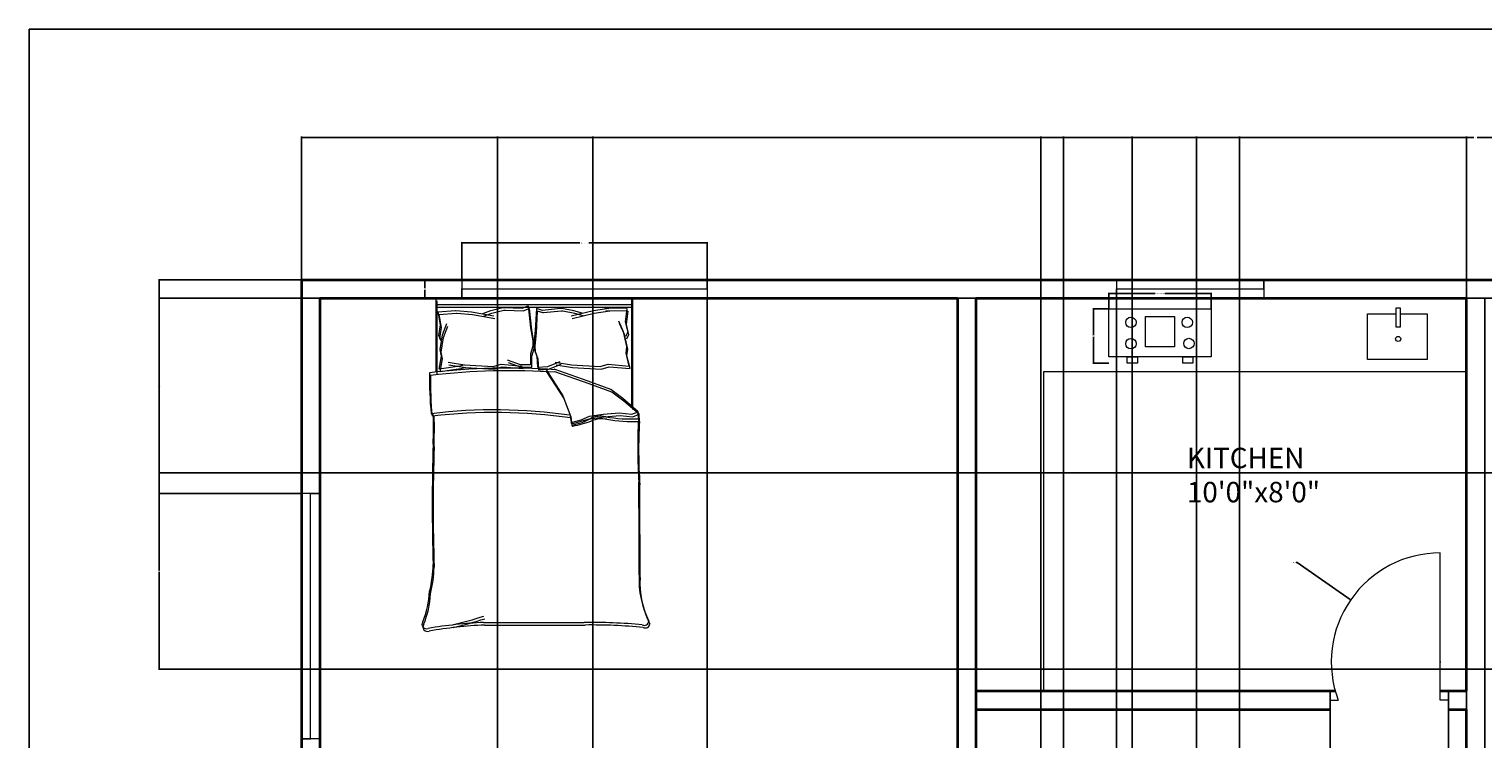
# Model space of a CAD drawing. Units: inches. Extents: x 1861 to 2564, y 1482 to 2317.
# Tile 7 of 11: x 1861 to 2217, y 2143 to 2317. Entities that reach past the tile are written whole.
import ezdxf

# ---------------------------------------------------------------- set-up
doc = ezdxf.new("R2010")
doc.units = ezdxf.units.IN
for name, color, linetype, lineweight in [('A-ANNO-DIMS', 2, 'Continuous', 18), ('A-ANNO-TTLB', 7, 'Continuous', 25), ('A-AREA-IDEN', 7, 'Continuous', 18), ('A-DOOR', 3, 'Continuous', 18), ('A-EQPM', 8, 'Continuous', 18), ('A-FLOR-CASE', 9, 'Continuous', 18), ('A-FLOR-FIXT', 8, 'Continuous', 18), ('A-FURN', 8, 'Continuous', 13), ('A-GLAZ', 4, 'Continuous', 18), ('A-WALL', 7, 'Continuous', 35)]:
    doc.layers.add(name, color=color, linetype=linetype, lineweight=lineweight)
doc.styles.get("Standard").update_dxf_attribs({"font": 'arial.ttf'})
doc.dimstyles.get("Standard").update_dxf_attribs({"dimtxt": 0.18, "dimasz": 0.18, "dimexe": 0.18, "dimexo": 0.0625, "dimgap": 0.09, "dimtad": 0, "dimtih": 1, "dimtoh": 1, "dimdec": 4, "dimzin": 0, "dimdsep": 46, "dimtxsty": 'Standard', "dimcen": 0.09, "dimadec": 0, "dimazin": 0, "dimtfac": 1, "dimtdec": 4, "dimtofl": 0, "dimtmove": 0, "dimatfit": 3, "dimfxl": 1, "dimtolj": 1, "dimtzin": 0, "dimarcsym": 0})

# ---------------------------------------------------------------- blocks, each defined once
blk = doc.blocks.new('WIN-60IN')
for p, q in [((0, 4.5), (0, 0)), ((60, 2.25), (60, 4.5)), ((60, 4.5), (60, 0)), ((0, 0), (0, 2.25)), ((0, 2.25), (60, 2.25))]:
    blk.add_line(p, q)
blk = doc.blocks.new('WIN-36IN')
for p, q in [((0, 4.5), (0, 0)), ((36, 2.25), (36, 4.5)), ((36, 4.5), (36, 0)), ((0, 0), (0, 2.25)), ((0, 2.25), (36, 2.25))]:
    blk.add_line(p, q)
blk = doc.blocks.new('BED-DOUBLE')
for p, q in [((3.48, 63.34), (3.48, 81.45)), ((3.48, 63.34), (3.48, 81.45)), ((51.27, 81.45), (3.48, 81.45)), ((3.48, 79.91), (51.27, 79.91)), ((3.48, 79.91), (51.27, 79.91)), ((3.7, 62.7), (3.7, 80.81)), ((3.7, 62.7), (3.7, 80.81)), ((3.7, 79.27), (51.49, 79.27)), ((3.7, 79.27), (51.49, 79.27)), ((3.9, 78.11), (8.18, 78.44)), ((3.9, 78.11), (8.18, 78.44)), ((8.18, 78.44), (8.29, 78.42)), ((8.18, 78.44), (8.29, 78.42)), ((8.29, 78.42), (12.11, 78.13)), ((8.29, 78.42), (12.11, 78.13)), ((14.86, 77.7), (16.88, 78.42)), ((14.86, 77.7), (16.88, 78.42)), ((16.88, 78.42), (19.77, 79.14)), ((16.88, 78.42), (19.77, 79.14)), ((17.11, 77.78), (20, 78.5)), ((17.11, 77.78), (20, 78.5)), ((19.77, 79.14), (20.09, 79.14)), ((19.77, 79.14), (20.09, 79.14)), ((20, 78.5), (20.32, 78.5)), ((20, 78.5), (20.32, 78.5)), ((20.09, 79.14), (24.54, 79)), ((20.09, 79.14), (24.54, 79)), ((20.32, 78.5), (24.77, 78.36)), ((20.32, 78.5), (24.77, 78.36)), ((24.54, 79), (25.98, 79.58)), ((24.54, 79), (25.98, 79.58)), ((24.77, 78.36), (26.21, 78.94)), ((24.77, 78.36), (26.21, 78.94)), ((25.98, 79.58), (26.56, 74.23)), ((25.98, 79.58), (26.56, 74.23)), ((26.21, 78.94), (26.79, 73.59)), ((26.21, 78.94), (26.79, 73.59)), ((27.98, 78.95), (27.73, 73.58)), ((27.98, 78.95), (27.73, 73.58)), ((28.21, 78.31), (27.96, 72.94)), ((28.21, 78.31), (27.96, 72.94)), ((29.46, 78.47), (27.98, 78.95)), ((29.46, 78.47), (27.98, 78.95)), ((29.69, 77.83), (28.21, 78.31)), ((29.68, 77.83), (28.21, 78.31)), ((33.88, 78.89), (29.46, 78.47)), ((33.88, 78.89), (29.46, 78.47)), ((34.11, 78.25), (29.68, 77.83)), ((34.11, 78.25), (29.69, 77.83)), ((34.21, 78.91), (33.88, 78.89)), ((34.21, 78.91), (33.88, 78.89)), ((34.43, 78.27), (34.11, 78.25)), ((34.43, 78.27), (34.11, 78.25)), ((37.14, 78.37), (34.21, 78.91)), ((37.14, 78.37), (34.21, 78.91)), ((37.36, 77.73), (34.43, 78.27)), ((37.36, 77.73), (34.43, 78.27)), ((41.92, 78.38), (36.5, 77.02)), ((41.92, 78.38), (36.5, 77.02)), ((39.2, 77.77), (37.14, 78.37)), ((39.2, 77.77), (37.14, 78.37)), ((45.71, 78.9), (41.92, 78.38)), ((45.71, 78.9), (41.92, 78.38)), ((45.94, 78.26), (42.14, 77.74)), ((45.94, 78.26), (42.14, 77.74)), ((50.11, 78.89), (44.71, 78.99)), ((44.71, 78.99), (45.71, 78.9)), ((50.11, 78.89), (44.71, 78.99)), ((44.71, 78.99), (45.71, 78.9)), ((50.34, 78.25), (44.94, 78.35)), ((44.94, 78.35), (45.94, 78.26)), ((50.34, 78.25), (44.94, 78.35)), ((44.94, 78.35), (45.94, 78.26)), ((50.11, 78.89), (49.73, 75.68)), ((50.11, 78.89), (49.73, 75.68)), ((50.34, 78.25), (49.96, 75.04)), ((50.34, 78.25), (49.96, 75.04)), ((51.27, 81.45), (51.27, 54.84)), ((51.27, 81.45), (51.27, 54.84)), ((51.27, 81.45), (51.49, 81.45)), ((51.49, 81.45), (51.49, 80.81)), ((51.49, 80.81), (51.49, 54.2)), ((51.49, 80.81), (51.49, 54.2)), ((3.9, 78.13), (4.47, 74.95)), ((3.9, 78.13), (4.47, 74.95)), ((4.47, 74.95), (4.04, 72.35)), ((4.47, 74.95), (4.04, 72.35)), ((4.12, 77.49), (4.7, 74.31)), ((4.12, 77.49), (4.7, 74.31)), ((4.13, 77.47), (8.41, 77.8)), ((4.13, 77.47), (8.41, 77.8)), ((5.05, 72.49), (6.06, 75.24)), ((5.05, 72.49), (6.06, 75.24)), ((8.41, 77.8), (8.51, 77.78)), ((8.41, 77.8), (8.51, 77.78)), ((8.51, 77.78), (12.34, 77.49)), ((8.51, 77.78), (12.34, 77.49)), ((12.11, 78.13), (17.6, 77.12)), ((12.11, 78.13), (17.6, 77.12)), ((12.34, 77.49), (17.83, 76.48)), ((12.34, 77.49), (17.83, 76.48)), ((15.08, 77.06), (17.11, 77.78)), ((15.08, 77.06), (17.11, 77.78)), ((42.14, 77.74), (36.72, 76.38)), ((42.14, 77.74), (36.72, 76.38)), ((39.43, 77.13), (37.36, 77.73)), ((39.43, 77.13), (37.36, 77.73)), ((49.31, 73.19), (48.13, 75.87)), ((49.31, 73.19), (48.13, 75.87)), ((49.54, 72.55), (48.36, 75.23)), ((49.54, 72.55), (48.36, 75.23)), ((49.73, 75.68), (50.33, 73.11)), ((49.73, 75.68), (50.33, 73.11)), ((49.96, 75.04), (50.56, 72.47)), ((49.96, 75.04), (50.56, 72.47)), ((4.04, 72.35), (4.62, 71.33)), ((4.04, 72.35), (4.62, 71.33)), ((4.7, 74.31), (4.27, 71.71)), ((4.7, 74.31), (4.27, 71.71)), ((4.27, 71.71), (4.85, 70.69)), ((4.27, 71.71), (4.85, 70.69)), ((4.47, 68.88), (5.05, 72.49)), ((4.47, 68.88), (5.05, 72.49)), ((4.7, 68.24), (5.28, 71.85)), ((4.7, 68.24), (5.28, 71.85)), ((5.28, 71.85), (6.29, 74.6)), ((5.28, 71.85), (6.29, 74.6)), ((26.56, 74.23), (27.14, 71.04)), ((26.56, 74.23), (27.14, 71.04)), ((26.79, 73.59), (27.37, 70.41)), ((26.79, 73.59), (27.37, 70.41)), ((27.73, 73.58), (27.36, 70.37)), ((27.73, 73.58), (27.36, 70.37)), ((27.96, 72.94), (27.58, 69.73)), ((27.96, 72.94), (27.58, 69.73)), ((50.11, 69.62), (49.31, 73.19)), ((50.11, 69.62), (49.31, 73.19)), ((50.34, 68.98), (49.54, 72.55)), ((50.34, 68.98), (49.54, 72.55)), ((50.33, 73.11), (49.82, 72.06)), ((50.33, 73.11), (49.82, 72.06)), ((50.56, 72.47), (50.04, 71.42)), ((50.56, 72.47), (50.04, 71.42)), ((4.76, 67.29), (4.47, 68.88)), ((4.76, 67.29), (4.47, 68.88)), ((4.99, 66.65), (4.7, 68.24)), ((4.99, 66.65), (4.7, 68.24)), ((27.14, 69.74), (26.56, 67.86)), ((27.14, 69.74), (26.56, 67.86)), ((26.56, 67.86), (26.56, 65.18)), ((26.56, 67.86), (26.56, 65.18)), ((27.37, 69.1), (26.79, 67.22)), ((27.37, 69.1), (26.79, 67.22)), ((27.14, 71.04), (27.14, 69.74)), ((27.14, 71.04), (27.14, 69.74)), ((27.36, 70.37), (27.44, 69.07)), ((27.36, 70.37), (27.44, 69.07)), ((27.37, 70.41), (27.37, 69.1)), ((27.37, 70.41), (27.37, 69.1)), ((27.44, 69.07), (28.13, 67.23)), ((27.44, 69.07), (28.13, 67.23)), ((27.58, 69.73), (27.67, 68.43)), ((27.58, 69.73), (27.67, 68.43)), ((27.67, 68.43), (28.36, 66.59)), ((27.67, 68.43), (28.36, 66.59)), ((49.92, 68.01), (50.11, 69.62)), ((49.92, 68.01), (50.11, 69.62)), ((50.7, 64.87), (49.92, 68.01)), ((50.7, 64.87), (49.92, 68.01)), ((50.15, 67.37), (50.34, 68.98)), ((50.15, 67.37), (50.34, 68.98)), ((4.18, 64.1), (4.76, 67.29)), ((4.18, 64.1), (4.76, 67.29)), ((9.28, 64.83), (4.18, 64.1)), ((9.28, 64.83), (4.18, 64.1)), ((4.41, 63.46), (4.99, 66.65)), ((4.41, 63.46), (4.99, 66.65)), ((9.51, 64.19), (4.41, 63.46)), ((9.51, 64.19), (4.41, 63.46)), ((6.38, 65.82), (10.41, 65.15)), ((6.38, 65.82), (10.41, 65.15)), ((6.61, 65.18), (10.64, 64.51)), ((6.61, 65.18), (10.64, 64.51)), ((10.41, 65.15), (9.28, 64.83)), ((10.41, 65.15), (9.28, 64.83)), ((10.64, 64.51), (9.51, 64.19)), ((10.64, 64.51), (9.51, 64.19)), ((10.41, 65.15), (17.42, 64.72)), ((10.41, 65.15), (17.42, 64.72)), ((10.64, 64.51), (17.65, 64.08)), ((10.64, 64.51), (17.65, 64.08)), ((17.42, 64.72), (19.38, 65.28)), ((17.42, 64.72), (19.38, 65.28)), ((17.65, 64.08), (19.61, 64.64)), ((17.65, 64.08), (19.61, 64.64)), ((19.38, 65.28), (24.52, 64.87)), ((19.38, 65.28), (24.52, 64.87)), ((19.61, 64.64), (24.75, 64.23)), ((19.61, 64.64), (24.74, 64.23)), ((24.1, 65.18), (20.96, 66.27)), ((24.1, 65.18), (20.96, 66.27)), ((24.33, 64.54), (21.19, 65.63)), ((24.33, 64.54), (21.19, 65.63)), ((26.56, 65.18), (24.1, 65.18)), ((26.56, 65.18), (24.1, 65.18)), ((26.79, 64.54), (24.33, 64.54)), ((26.79, 64.54), (24.33, 64.54)), ((26.79, 67.22), (26.79, 64.54)), ((26.79, 67.22), (26.79, 64.54)), ((28.13, 67.23), (28.3, 64.55)), ((28.13, 67.23), (28.3, 64.55)), ((28.3, 64.55), (30.75, 64.71)), ((28.3, 64.55), (30.75, 64.71)), ((28.36, 66.59), (28.53, 63.91)), ((28.36, 66.59), (28.53, 63.91)), ((28.53, 63.91), (30.98, 64.07)), ((28.53, 63.91), (30.98, 64.07)), ((30.26, 64.06), (34.45, 57.57)), ((30.26, 64.06), (34.45, 57.57)), ((30.75, 64.71), (33.82, 65.99)), ((30.75, 64.71), (33.82, 65.99)), ((30.98, 64.07), (34.05, 65.35)), ((30.98, 64.07), (34.05, 65.35)), ((40.65, 61.13), (32.31, 64.06)), ((40.64, 61.13), (32.31, 64.06)), ((32.56, 65.82), (36.6, 65.15)), ((32.57, 65.82), (36.6, 65.15)), ((32.79, 65.18), (36.83, 64.51)), ((32.79, 65.18), (36.83, 64.51)), ((36.6, 65.15), (43.61, 64.72)), ((36.6, 65.15), (43.61, 64.72)), ((36.83, 64.51), (43.84, 64.08)), ((36.83, 64.51), (43.84, 64.08)), ((43.61, 64.72), (45.57, 65.28)), ((43.61, 64.72), (45.57, 65.28)), ((43.84, 64.08), (45.8, 64.64)), ((43.84, 64.08), (45.8, 64.64)), ((45.57, 65.28), (50.7, 64.87)), ((45.57, 65.28), (50.7, 64.87)), ((45.8, 64.64), (50.93, 64.23)), ((45.8, 64.64), (50.93, 64.23)), ((50.93, 64.23), (50.15, 67.37)), ((50.93, 64.23), (50.15, 67.37)), ((30.49, 63.42), (34.68, 56.93)), ((30.49, 63.42), (34.68, 56.93)), ((40.87, 60.49), (32.54, 63.42)), ((40.87, 60.49), (32.54, 63.42)), ((46.22, 59.12), (40.64, 61.13)), ((46.22, 59.12), (40.65, 61.13)), ((46.45, 58.48), (40.87, 60.49)), ((46.45, 58.48), (40.87, 60.49)), ((34.45, 57.57), (36.15, 53.08)), ((34.45, 57.57), (36.15, 53.08)), ((34.68, 56.93), (36.38, 52.44)), ((34.68, 56.93), (36.38, 52.44)), ((49.16, 56.95), (46.22, 59.12)), ((49.16, 56.95), (46.22, 59.12)), ((49.39, 56.31), (46.45, 58.48)), ((49.39, 56.31), (46.45, 58.48)), ((52.87, 53.7), (49.16, 56.95)), ((52.87, 53.7), (49.16, 56.95)), ((44.36, 53.08), (48.23, 53.39)), ((44.36, 53.08), (48.23, 53.39)), ((48.23, 53.39), (51.33, 53.08)), ((48.23, 53.39), (51.33, 53.08)), ((53.1, 53.06), (49.39, 56.31)), ((53.1, 53.06), (49.39, 56.31)), ((51.33, 53.08), (52.87, 53.7)), ((51.33, 53.08), (52.87, 53.7)), ((52.95, 51.95), (52.87, 53.7, 3.87)), ((52.95, 51.95), (52.87, 53.7, 3.87)), ((36.15, 53.08), (36.46, 51.07)), ((36.15, 53.08), (36.46, 51.07)), ((36.38, 52.44), (36.69, 50.43)), ((36.38, 52.44), (36.69, 50.43)), ((36.46, 51.07), (38.94, 51.69)), ((36.46, 51.07), (38.94, 51.69)), ((36.69, 50.43), (39.17, 51.05)), ((36.69, 50.43), (39.17, 51.05)), ((38.94, 51.69), (40.95, 52.62)), ((38.94, 51.69), (40.95, 52.62)), ((39.17, 51.05), (41.18, 51.98)), ((39.17, 51.05), (41.18, 51.98)), ((40.95, 52.62), (44.36, 53.08)), ((40.95, 52.62), (44.36, 53.08)), ((41.18, 51.98), (44.59, 52.44)), ((41.18, 51.98), (44.59, 52.44)), ((44.59, 52.44), (48.46, 52.75)), ((44.59, 52.44), (48.46, 52.75)), ((48.46, 52.75), (51.56, 52.44)), ((48.46, 52.75), (51.56, 52.44)), ((51.56, 52.44), (53.1, 53.06)), ((51.56, 52.44), (53.1, 53.06)), ((53.18, 51.32), (53.1, 53.06, 3.87)), ((53.18, 51.32), (53.1, 53.06, 3.87)), ((15.06, 2.2), (39.68, 2.2)), ((15.06, 2.2), (39.68, 2.2)), ((15.29, 1.56), (39.91, 1.56)), ((15.29, 1.56), (39.91, 1.56))]:
    blk.add_line(p, q)
for centre, radius, start, end in [((21.36, -100.61), 164.97, 86.0865, 96.7821), ((21.36, -100.61), 164.97, 86.0865, 96.7821), ((85.16, 61.35), 83.31, 178.7218, 185.604), ((85.16, 61.35), 83.31, 178.7218, 185.604), ((85.39, 60.71), 83.31, 178.7218, 185.604), ((85.39, 60.71), 83.31, 178.7218, 185.604), ((21.59, -101.25), 164.97, 86.0865, 96.7821), ((21.59, -101.25), 164.97, 86.0865, 96.7821), ((17.76, -74.87), 129.02, 81.7845, 96.9006), ((17.76, -74.87), 129.02, 81.7845, 96.9006), ((17.99, -75.51), 129.02, 81.7845, 96.9006), ((17.98, -75.51), 129.02, 81.7845, 96.9006), ((-167.31, 50.27), 170.11, 358.4762, 1.0082), ((-167.31, 50.27), 170.11, 358.4762, 1.0082), ((-167.08, 49.63), 170.11, 358.4762, 1.0082), ((-167.08, 49.63), 170.11, 358.4762, 1.0082), ((36.64, 51.01), 0.185, 160.2464, 271.1377), ((36.64, 51.01), 0.185, 160.2464, 271.1377), ((31.15, 79.96), 29.65, 280.6617, 289.8806), ((31.15, 79.96), 29.65, 280.6617, 289.8806), ((36.87, 50.37), 0.185, 160.2464, 271.1377), ((36.87, 50.37), 0.185, 160.2464, 271.1377), ((31.38, 79.32), 29.65, 280.6617, 289.8806), ((31.38, 79.32), 29.65, 280.6617, 289.8806), ((43.74, 46.38), 6.22, 78.6608, 113.7384), ((43.74, 46.38), 6.22, 78.6608, 113.7384), ((43.97, 45.74), 6.22, 78.6608, 113.7384), ((43.97, 45.74), 6.22, 78.6608, 113.7384), ((51.33, 88.1), 36.18, 259.8763, 272.5657), ((51.33, 88.1), 36.18, 259.8763, 272.5657), ((51.56, 87.46), 36.18, 259.8763, 272.5657), ((51.56, 87.46), 36.18, 259.8763, 272.5657), ((182.27, 45.13), 129.5, 176.9791, 183.8365), ((182.27, 45.13), 129.5, 176.9791, 183.8365), ((182.5, 44.49), 129.5, 176.9791, 183.8365), ((182.49, 44.49), 129.5, 176.9791, 183.8365), ((484.82, 30.83), 482.31, 178.2277, 181.7185), ((484.82, 30.83), 482.31, 178.2277, 181.7185), ((485.05, 30.19), 482.31, 178.2277, 181.7185), ((485.05, 30.19), 482.31, 178.2277, 181.7185), ((-4508.74, 13.62), 4561.86, 0.00217, 0.28689), ((-4508.74, 13.62), 4561.86, 0.00217, 0.28689), ((-4508.51, 12.98), 4561.86, 0.00217, 0.28689), ((-4508.51, 12.98), 4561.86, 0.00217, 0.28689), ((-26.9, 16.93), 29.63, 346.0648, 358.9113), ((-26.9, 16.93), 29.63, 346.0648, 358.9113), ((-26.67, 16.29), 29.63, 346.0648, 358.9113), ((-26.67, 16.29), 29.63, 346.0648, 358.9113), ((76.16, 12.78), 23.07, 177.4714, 206.4681), ((76.16, 12.78), 23.07, 177.4714, 206.4681), ((76.39, 12.14), 23.07, 177.4714, 206.4681), ((76.39, 12.14), 23.07, 177.4714, 206.4681), ((-21.66, 11.17), 23.56, 337.9751, 356.652), ((-21.66, 11.17), 23.56, 337.9751, 356.652), ((-21.43, 10.53), 23.56, 337.9751, 356.652), ((-21.43, 10.53), 23.56, 337.9751, 356.652), ((-17.22, 105.16), 106.46, 283.3832, 287.7053), ((-17.22, 105.16), 106.46, 283.3832, 287.7053), ((1.09, 1.73), 1.09, 146.1736, 293.4781), ((1.09, 1.73), 1.09, 146.1736, 293.4781), ((1.32, 1.09), 1.09, 146.1736, 293.4781), ((1.32, 1.09), 1.09, 146.1736, 293.4781), ((21.43, -119.39), 121.76, 92.9958, 99.4091), ((21.43, -119.39), 121.76, 92.9958, 99.4091), ((21.66, -120.03), 121.76, 92.9958, 99.4091), ((21.66, -120.03), 121.76, 92.9958, 99.4091), ((-16.99, 104.52), 106.46, 283.3832, 287.7053), ((-16.99, 104.52), 106.46, 283.3832, 287.7053), ((41.15, -130.83), 133.04, 84.4998, 90.6351), ((41.15, -130.83), 133.04, 84.4998, 90.6351), ((41.38, -131.47), 133.04, 84.4998, 90.6351), ((41.38, -131.47), 133.04, 84.4998, 90.6351), ((54.41, 2.58), 1.1, 242.6588, 356.02), ((54.41, 2.58), 1.1, 242.6588, 356.02), ((54.64, 1.94), 1.1, 242.6588, 356.02), ((54.64, 1.94), 1.1, 242.6588, 356.02)]:
    blk.add_arc(centre, radius, start, end)
blk = doc.blocks.new('SINK-KITCHEN')
blk.add_lwpolyline([(7.97, 11.14), (14.59, 11.14), (14.59, 0), (0, 0), (0, 11.14), (6.99, 11.14)])
blk.add_lwpolyline([(6.99, 12.66), (7.97, 12.66), (7.97, 7.92), (6.99, 7.92)], close=True)
blk.add_circle((7.5, 5.01), 0.628)
blk = doc.blocks.new('COOKTOP-4B')
for points in [[(-0.01, 13.28), (25.01, 13.28), (25.01, 1.58), (-0.01, 1.58)], [(8.91, 11.43), (16.01, 11.43), (16.01, 4.05), (8.91, 4.05)], [(4.47, 1.58), (6.95, 1.58), (6.95, 0), (4.47, 0)], [(18.04, 1.58), (20.51, 1.58), (20.51, 0), (18.04, 0)]]:
    blk.add_lwpolyline(points, close=True)
for centre in [(5.36, 10), (19.16, 10), (5.36, 4.79), (19.56, 4.83)]:
    blk.add_circle(centre, 1.27)
blk = doc.blocks.new('*D20')
at = {"layer": 'A-ANNO-DIMS', "color": 0, "lineweight": -2, "transparency": 16777216}
for p, q in [((1966.99, 2255.45), (1966.99, 2264.57)), ((1967.17, 2264.39), (1995.87, 2264.39)), ((2026.81, 2264.39), (1998.11, 2264.39)), ((2026.99, 2255.45), (2026.99, 2264.57))]:
    blk.add_line(p, q, dxfattribs=at)
at = {"layer": 'A-ANNO-DIMS', "color": 0, "transparency": 16777216}
for points in [[(1967.17, 2264.42), (1967.17, 2264.36), (1966.99, 2264.39)], [(2026.81, 2264.42), (2026.81, 2264.36), (2026.99, 2264.39)]]:
    blk.add_solid(points, dxfattribs=at)
at = {"layer": 'Defpoints', "color": 0, "transparency": 16777216}
for p in [(2026.99, 2264.39), (1966.99, 2255.39), (2026.99, 2255.39)]:
    blk.add_point(p, dxfattribs=at)
at = {"layer": 'A-ANNO-DIMS', "color": 0, "transparency": 16777216, "insert": (1996.99, 2264.39), "char_height": 0.18, "attachment_point": 5}
blk.add_mtext('\\A1;WINDOW 60 TYP.', dxfattribs=at)
blk = doc.blocks.new('*D21')
at = {"layer": 'A-ANNO-DIMS', "color": 0, "lineweight": -2, "transparency": 16777216}
for p, q in [((1966.93, 2255.39), (1957.81, 2255.39)), ((1957.99, 2255.21), (1957.99, 2253.32)), ((1957.99, 2251.07), (1957.99, 2252.95)), ((1966.93, 2250.89), (1957.81, 2250.89))]:
    blk.add_line(p, q, dxfattribs=at)
at = {"layer": 'A-ANNO-DIMS', "color": 0, "transparency": 16777216}
for points in [[(1957.96, 2255.21), (1958.02, 2255.21), (1957.99, 2255.39)], [(1957.96, 2251.07), (1958.02, 2251.07), (1957.99, 2250.89)]]:
    blk.add_solid(points, dxfattribs=at)
at = {"layer": 'Defpoints', "color": 0, "transparency": 16777216}
for p in [(1957.99, 2255.39), (1966.99, 2255.39), (1966.99, 2250.89)]:
    blk.add_point(p, dxfattribs=at)
at = {"layer": 'A-ANNO-DIMS', "color": 0, "transparency": 16777216, "insert": (1957.99, 2253.14), "char_height": 0.18, "attachment_point": 5}
blk.add_mtext('\\A1;5 TYP.', dxfattribs=at)
blk = doc.blocks.new('*D24')
at = {"layer": 'A-ANNO-DIMS', "color": 0, "lineweight": -2, "transparency": 16777216}
for p, q in [((2125.31, 2248.33), (2125.31, 2252.2)), ((2125.49, 2252.02), (2136.63, 2252.02)), ((2150.15, 2252.02), (2139.01, 2252.02)), ((2150.33, 2248.33), (2150.33, 2252.2))]:
    blk.add_line(p, q, dxfattribs=at)
at = {"layer": 'A-ANNO-DIMS', "color": 0, "transparency": 16777216}
for points in [[(2125.49, 2252.05), (2125.49, 2251.99), (2125.31, 2252.02)], [(2150.15, 2252.05), (2150.15, 2251.99), (2150.33, 2252.02)]]:
    blk.add_solid(points, dxfattribs=at)
at = {"layer": 'Defpoints', "color": 0, "transparency": 16777216}
for p in [(2150.33, 2252.02), (2125.31, 2248.26), (2150.33, 2248.26)]:
    blk.add_point(p, dxfattribs=at)
at = {"layer": 'A-ANNO-DIMS', "color": 0, "transparency": 16777216, "insert": (2137.82, 2252.02), "char_height": 0.18, "attachment_point": 5}
blk.add_mtext('\\A1;COOKTOP 25 TYP.', dxfattribs=at)
blk = doc.blocks.new('*D25')
at = {"layer": 'A-ANNO-DIMS', "color": 0, "lineweight": -2, "transparency": 16777216}
for p, q in [((2125.25, 2248.26), (2121.38, 2248.26)), ((2121.56, 2248.08), (2121.56, 2241.81)), ((2121.56, 2235.16), (2121.56, 2241.44)), ((2125.25, 2234.98), (2121.38, 2234.98))]:
    blk.add_line(p, q, dxfattribs=at)
at = {"layer": 'A-ANNO-DIMS', "color": 0, "transparency": 16777216}
for points in [[(2121.53, 2248.08), (2121.59, 2248.08), (2121.56, 2248.26)], [(2121.53, 2235.16), (2121.59, 2235.16), (2121.56, 2234.98)]]:
    blk.add_solid(points, dxfattribs=at)
at = {"layer": 'Defpoints', "color": 0, "transparency": 16777216}
for p in [(2121.56, 2248.26), (2125.31, 2248.26), (2125.31, 2234.98)]:
    blk.add_point(p, dxfattribs=at)
at = {"layer": 'A-ANNO-DIMS', "color": 0, "transparency": 16777216, "insert": (2121.56, 2241.62), "char_height": 0.18, "attachment_point": 5}
blk.add_mtext('\\A1;13 TYP.', dxfattribs=at)
blk = doc.blocks.new('*D34')
at = {"layer": 'A-ANNO-DIMS', "color": 0, "lineweight": -2, "transparency": 16777216}
for p, q in [((1927.74, 2255.45), (1927.74, 2290.37)), ((1927.92, 2290.19), (2214.59, 2290.19)), ((2502.06, 2290.19), (2215.38, 2290.19)), ((2502.24, 2255.45), (2502.24, 2290.37))]:
    blk.add_line(p, q, dxfattribs=at)
at = {"layer": 'A-ANNO-DIMS', "color": 0, "transparency": 16777216}
for points in [[(1927.92, 2290.22), (1927.92, 2290.16), (1927.74, 2290.19)], [(2502.06, 2290.22), (2502.06, 2290.16), (2502.24, 2290.19)]]:
    blk.add_solid(points, dxfattribs=at)
at = {"layer": 'Defpoints', "color": 0, "transparency": 16777216}
for p in [(2502.24, 2290.19), (1927.74, 2255.39), (2502.24, 2255.39)]:
    blk.add_point(p, dxfattribs=at)
at = {"layer": 'A-ANNO-DIMS', "color": 0, "transparency": 16777216, "insert": (2214.99, 2290.19), "char_height": 0.18, "attachment_point": 5}
blk.add_mtext('\\A1;574.5', dxfattribs=at)
blk = doc.blocks.new('*D35')
at = {"layer": 'A-ANNO-DIMS', "color": 0, "lineweight": -2, "transparency": 16777216}
for p, q in [((2026.99, 2250.82), (2026.99, 1545.6)), ((2088.24, 2250.82), (2088.24, 1545.6)), ((2027.17, 1545.78), (2057.22, 1545.78)), ((2088.06, 1545.78), (2058.01, 1545.78))]:
    blk.add_line(p, q, dxfattribs=at)
at = {"layer": 'A-ANNO-DIMS', "color": 0, "transparency": 16777216}
for points in [[(2027.17, 1545.81), (2027.17, 1545.75), (2026.99, 1545.78)], [(2088.06, 1545.81), (2088.06, 1545.75), (2088.24, 1545.78)]]:
    blk.add_solid(points, dxfattribs=at)
at = {"layer": 'Defpoints', "color": 0, "transparency": 16777216}
for p in [(2026.99, 2250.89), (2088.24, 2250.89), (2088.24, 1545.78)]:
    blk.add_point(p, dxfattribs=at)
at = {"layer": 'A-ANNO-DIMS', "color": 0, "transparency": 16777216, "insert": (2057.61, 1545.78), "char_height": 0.18, "attachment_point": 5}
blk.add_mtext('\\A1;61.25', dxfattribs=at)
blk = doc.blocks.new('*D36')
at = {"layer": 'A-ANNO-DIMS', "color": 0, "lineweight": -2, "transparency": 16777216}
for p, q in [((2092.74, 2250.82), (2092.74, 1545.6)), ((2127.18, 2250.82), (2127.18, 1545.6)), ((2092.92, 1545.78), (2109.5, 1545.78)), ((2127, 1545.78), (2110.43, 1545.78))]:
    blk.add_line(p, q, dxfattribs=at)
at = {"layer": 'A-ANNO-DIMS', "color": 0, "transparency": 16777216}
for points in [[(2092.92, 1545.81), (2092.92, 1545.75), (2092.74, 1545.78)], [(2127, 1545.81), (2127, 1545.75), (2127.18, 1545.78)]]:
    blk.add_solid(points, dxfattribs=at)
at = {"layer": 'Defpoints', "color": 0, "transparency": 16777216}
for p in [(2092.74, 2250.89), (2127.18, 2250.89), (2127.18, 1545.78)]:
    blk.add_point(p, dxfattribs=at)
at = {"layer": 'A-ANNO-DIMS', "color": 0, "transparency": 16777216, "insert": (2109.96, 1545.78), "char_height": 0.18, "attachment_point": 5}
blk.add_mtext('\\A1;34.445', dxfattribs=at)
blk = doc.blocks.new('*D39')
at = {"layer": 'A-ANNO-DIMS', "color": 0, "lineweight": -2, "transparency": 16777216}
for p, q in [((1927.68, 2255.39), (1892.76, 2255.39)), ((1892.94, 2255.21), (1892.94, 2229.46)), ((1892.94, 2203.35), (1892.94, 2229.09)), ((1927.68, 2203.17), (1892.76, 2203.17))]:
    blk.add_line(p, q, dxfattribs=at)
at = {"layer": 'A-ANNO-DIMS', "color": 0, "transparency": 16777216}
for points in [[(1892.91, 2255.21), (1892.97, 2255.21), (1892.94, 2255.39)], [(1892.91, 2203.35), (1892.97, 2203.35), (1892.94, 2203.17)]]:
    blk.add_solid(points, dxfattribs=at)
at = {"layer": 'Defpoints', "color": 0, "transparency": 16777216}
for p in [(1927.74, 2255.39), (1892.94, 2203.17), (1927.74, 2203.17)]:
    blk.add_point(p, dxfattribs=at)
at = {"layer": 'A-ANNO-DIMS', "color": 0, "transparency": 16777216, "insert": (1892.94, 2229.28), "char_height": 0.18, "attachment_point": 5}
blk.add_mtext('\\A1;52.22', dxfattribs=at)
blk = doc.blocks.new('*D52')
at = {"layer": 'A-ANNO-DIMS', "color": 0, "lineweight": -2, "transparency": 16777216}
for p, q in [((2179.39, 2154.82), (2179.39, 1545.6)), ((2208.37, 2154.82), (2208.37, 1545.6)), ((2179.57, 1545.78), (2193.49, 1545.78)), ((2208.19, 1545.78), (2194.28, 1545.78))]:
    blk.add_line(p, q, dxfattribs=at)
at = {"layer": 'A-ANNO-DIMS', "color": 0, "transparency": 16777216}
for points in [[(2179.57, 1545.81), (2179.57, 1545.75), (2179.39, 1545.78)], [(2208.19, 1545.81), (2208.19, 1545.75), (2208.37, 1545.78)]]:
    blk.add_solid(points, dxfattribs=at)
at = {"layer": 'Defpoints', "color": 0, "transparency": 16777216}
for p in [(2179.39, 2154.89), (2208.37, 2154.89), (2208.37, 1545.78)]:
    blk.add_point(p, dxfattribs=at)
at = {"layer": 'A-ANNO-DIMS', "color": 0, "transparency": 16777216, "insert": (2193.88, 1545.78), "char_height": 0.18, "attachment_point": 5}
blk.add_mtext('\\A1;28.98', dxfattribs=at)
blk = doc.blocks.new('*D54')
at = {"layer": 'A-ANNO-DIMS', "color": 0, "lineweight": -2, "transparency": 16777216}
for p, q in [((1975.71, 1905.95), (1975.71, 2290.37)), ((1975.89, 2290.19), (1986.91, 2290.19)), ((1998.87, 2290.19), (1987.85, 2290.19)), ((1999.05, 1905.95), (1999.05, 2290.37))]:
    blk.add_line(p, q, dxfattribs=at)
at = {"layer": 'A-ANNO-DIMS', "color": 0, "transparency": 16777216}
for points in [[(1975.89, 2290.22), (1975.89, 2290.16), (1975.71, 2290.19)], [(1998.87, 2290.22), (1998.87, 2290.16), (1999.05, 2290.19)]]:
    blk.add_solid(points, dxfattribs=at)
at = {"layer": 'Defpoints', "color": 0, "transparency": 16777216}
for p in [(1999.05, 2290.19), (1975.71, 1905.89), (1999.05, 1905.89)]:
    blk.add_point(p, dxfattribs=at)
at = {"layer": 'A-ANNO-DIMS', "color": 0, "transparency": 16777216, "insert": (1987.38, 2290.19), "char_height": 0.18, "attachment_point": 5}
blk.add_mtext('\\A1;23.335', dxfattribs=at)
blk = doc.blocks.new('*D55')
at = {"layer": 'A-ANNO-DIMS', "color": 0, "lineweight": -2, "transparency": 16777216}
for p, q in [((2114.18, 1853.45), (2114.18, 2290.37)), ((2114.36, 2290.19), (2130, 2290.19)), ((2146.56, 2290.19), (2130.92, 2290.19)), ((2146.74, 1853.45), (2146.74, 2290.37))]:
    blk.add_line(p, q, dxfattribs=at)
at = {"layer": 'A-ANNO-DIMS', "color": 0, "transparency": 16777216}
for points in [[(2114.36, 2290.22), (2114.36, 2290.16), (2114.18, 2290.19)], [(2146.56, 2290.22), (2146.56, 2290.16), (2146.74, 2290.19)]]:
    blk.add_solid(points, dxfattribs=at)
at = {"layer": 'Defpoints', "color": 0, "transparency": 16777216}
for p in [(2146.74, 2290.19), (2114.18, 1853.39), (2146.74, 1853.39)]:
    blk.add_point(p, dxfattribs=at)
at = {"layer": 'A-ANNO-DIMS', "color": 0, "transparency": 16777216, "insert": (2130.46, 2290.19), "char_height": 0.18, "attachment_point": 5}
blk.add_mtext('\\A1;32.564', dxfattribs=at)
blk = doc.blocks.new('*D60')
at = {"layer": 'A-ANNO-DIMS', "color": 0, "lineweight": -2, "transparency": 16777216}
for p, q in [((2497.68, 2208.17), (1892.76, 2208.17)), ((1892.94, 2207.99), (1892.94, 2184.35)), ((1892.94, 2160.35), (1892.94, 2183.99)), ((2497.68, 2160.17), (1892.76, 2160.17))]:
    blk.add_line(p, q, dxfattribs=at)
at = {"layer": 'A-ANNO-DIMS', "color": 0, "transparency": 16777216}
for points in [[(1892.91, 2207.99), (1892.97, 2207.99), (1892.94, 2208.17)], [(1892.91, 2160.35), (1892.97, 2160.35), (1892.94, 2160.17)]]:
    blk.add_solid(points, dxfattribs=at)
at = {"layer": 'Defpoints', "color": 0, "transparency": 16777216}
for p in [(1892.94, 2208.17), (2497.74, 2208.17), (2497.74, 2160.17)]:
    blk.add_point(p, dxfattribs=at)
at = {"layer": 'A-ANNO-DIMS', "color": 0, "transparency": 16777216, "insert": (1892.94, 2184.17), "char_height": 0.18, "attachment_point": 5}
blk.add_mtext('\\A1;48', dxfattribs=at)
blk = doc.blocks.new('*D62')
at = {"layer": 'A-ANNO-DIMS', "color": 0, "lineweight": -2, "transparency": 16777216}
for p, q in [((2108.68, 1781.45), (2108.68, 2290.37)), ((2108.86, 2290.19), (2119.46, 2290.19)), ((2130.84, 2290.19), (2120.25, 2290.19)), ((2131.02, 1781.45), (2131.02, 2290.37))]:
    blk.add_line(p, q, dxfattribs=at)
at = {"layer": 'A-ANNO-DIMS', "color": 0, "transparency": 16777216}
for points in [[(2108.86, 2290.22), (2108.86, 2290.16), (2108.68, 2290.19)], [(2130.84, 2290.22), (2130.84, 2290.16), (2131.02, 2290.19)]]:
    blk.add_solid(points, dxfattribs=at)
at = {"layer": 'Defpoints', "color": 0, "transparency": 16777216}
for p in [(2131.02, 2290.19), (2108.68, 1781.39), (2131.02, 1781.39)]:
    blk.add_point(p, dxfattribs=at)
at = {"layer": 'A-ANNO-DIMS', "color": 0, "transparency": 16777216, "insert": (2119.85, 2290.19), "char_height": 0.18, "attachment_point": 5}
blk.add_mtext('\\A1;22.34', dxfattribs=at)
blk = doc.blocks.new('*D63')
at = {"layer": 'A-ANNO-DIMS', "color": 0, "lineweight": -2, "transparency": 16777216}
for p, q in [((2497.68, 2250.89), (1892.76, 2250.89)), ((1892.94, 2250.71), (1892.94, 2229.71)), ((1892.94, 2208.35), (1892.94, 2229.35)), ((2497.68, 2208.17), (1892.76, 2208.17))]:
    blk.add_line(p, q, dxfattribs=at)
at = {"layer": 'A-ANNO-DIMS', "color": 0, "transparency": 16777216}
for points in [[(1892.91, 2250.71), (1892.97, 2250.71), (1892.94, 2250.89)], [(1892.91, 2208.35), (1892.97, 2208.35), (1892.94, 2208.17)]]:
    blk.add_solid(points, dxfattribs=at)
at = {"layer": 'Defpoints', "color": 0, "transparency": 16777216}
for p in [(2497.74, 2250.89), (1892.94, 2208.17), (2497.74, 2208.17)]:
    blk.add_point(p, dxfattribs=at)
at = {"layer": 'A-ANNO-DIMS', "color": 0, "transparency": 16777216, "insert": (1892.94, 2229.53), "char_height": 0.18, "attachment_point": 5}
blk.add_mtext('\\A1;42.71', dxfattribs=at)
blk = doc.blocks.new('*D68')
at = {"layer": 'A-ANNO-DIMS', "color": 0, "lineweight": -2, "transparency": 16777216}
for p, q in [((2157.24, 1794.95), (2157.24, 2290.37)), ((2157.42, 2290.19), (2184.66, 2290.19)), ((2212.56, 2290.19), (2185.31, 2290.19)), ((2212.74, 1794.95), (2212.74, 2290.37))]:
    blk.add_line(p, q, dxfattribs=at)
at = {"layer": 'A-ANNO-DIMS', "color": 0, "transparency": 16777216}
for points in [[(2157.42, 2290.22), (2157.42, 2290.16), (2157.24, 2290.19)], [(2212.56, 2290.22), (2212.56, 2290.16), (2212.74, 2290.19)]]:
    blk.add_solid(points, dxfattribs=at)
at = {"layer": 'Defpoints', "color": 0, "transparency": 16777216}
for p in [(2212.74, 2290.19), (2157.24, 1794.89), (2212.74, 1794.89)]:
    blk.add_point(p, dxfattribs=at)
at = {"layer": 'A-ANNO-DIMS', "color": 0, "transparency": 16777216, "insert": (2184.99, 2290.19), "char_height": 0.18, "attachment_point": 5}
blk.add_mtext('\\A1;55.5', dxfattribs=at)
blk = doc.blocks.new('*D71')
at = {"layer": 'A-ANNO-DIMS', "color": 0, "lineweight": -2, "transparency": 16777216}
for p, q in [((2212.74, 2250.82), (2212.74, 1545.6)), ((2217.24, 2250.82), (2217.24, 1545.6)), ((2212.92, 1545.78), (2214.73, 1545.78)), ((2217.06, 1545.78), (2215.25, 1545.78))]:
    blk.add_line(p, q, dxfattribs=at)
at = {"layer": 'A-ANNO-DIMS', "color": 0, "transparency": 16777216}
for points in [[(2212.92, 1545.81), (2212.92, 1545.75), (2212.74, 1545.78)], [(2217.06, 1545.81), (2217.06, 1545.75), (2217.24, 1545.78)]]:
    blk.add_solid(points, dxfattribs=at)
at = {"layer": 'Defpoints', "color": 0, "transparency": 16777216}
for p in [(2212.74, 2250.89), (2217.24, 2250.89), (2217.24, 1545.78)]:
    blk.add_point(p, dxfattribs=at)
at = {"layer": 'A-ANNO-DIMS', "color": 0, "transparency": 16777216, "insert": (2214.99, 1545.78), "char_height": 0.18, "attachment_point": 5}
blk.add_mtext('\\A1;4.5', dxfattribs=at)
blk = doc.blocks.new('*D83')
at = {"layer": 'A-ANNO-DIMS', "color": 0, "lineweight": -2, "transparency": 16777216}
for p, q in [((2171.14, 2186.29), (2171.32, 2186.29)), ((2171.32, 2186.29), (2184.32, 2177.27)), ((2206.28, 2161.97), (2206.46, 2161.97)), ((2206.37, 2161.88), (2206.37, 2162.06))]:
    blk.add_line(p, q, dxfattribs=at)
at = {"layer": 'A-ANNO-DIMS', "color": 0, "transparency": 16777216}
blk.add_solid([(2184.33, 2177.3), (2184.3, 2177.25), (2184.46, 2177.17)], dxfattribs=at)
at = {"layer": 'Defpoints', "color": 0, "transparency": 16777216}
for p in [(2184.46, 2177.17), (2206.37, 2161.97)]:
    blk.add_point(p, dxfattribs=at)
at = {"layer": 'A-ANNO-DIMS', "color": 0, "transparency": 16777216, "insert": (2170.66, 2186.29), "char_height": 0.18, "attachment_point": 5}
blk.add_mtext('\\A1;R26.67', dxfattribs=at)

msp = doc.modelspace()

# ---------------------------------------------------------------- linework, layer by layer
at = {"layer": 'A-ANNO-TTLB'}
msp.add_lwpolyline([(1861.1332, 2316.6589), (2563.8077, 2316.6589), (2563.8077, 1482.0728), (1861.1332, 1482.0728)], close=True, dxfattribs=at)
at = {"layer": 'A-DOOR'}
for p, q in [((2206.3728, 2152.6354), (2206.3728, 2188.6354)), ((2179.3907, 2154.8854), (2179.3907, 2150.3854)), ((2179.3907, 2150.3854), (2179.3907, 2152.6354)), ((2179.3907, 2152.6354), (2181.3907, 2152.6354)), ((2208.3728, 2152.6354), (2206.3728, 2152.6354)), ((2208.3728, 2154.8854), (2208.3728, 2150.3854)), ((2208.3728, 2150.3854), (2208.3728, 2152.6354))]:
    msp.add_line(p, q, dxfattribs=at)
msp.add_arc((2206.3728, 2161.9673), 26.6681, 90, 200.482864, dxfattribs=at)
at = {"layer": 'A-FLOR-CASE'}
for p, q in [((2109.3866, 2154.8854), (2109.3866, 2232.9509)), ((2109.3866, 2232.9509), (2212.7393, 2232.9509))]:
    msp.add_line(p, q, dxfattribs=at)
at = {"layer": 'A-WALL'}
for p, q in [((1927.7393, 2255.3854), (2502.2393, 2255.3854)), ((1927.7393, 2255.3854), (1927.7393, 1700.3854)), ((1932.2393, 2250.8854), (2088.2393, 2250.8854)), ((1932.2393, 2250.8854), (1932.2393, 2106.8854)), ((2088.2393, 2250.8854), (2088.2393, 2106.8854)), ((2092.7393, 2250.8854), (2092.7393, 2102.3854)), ((2092.7393, 2250.8854), (2212.7393, 2250.8854)), ((2212.7393, 2250.8854), (2212.7393, 2154.8854)), ((2092.7393, 2154.8854), (2180.6622, 2154.8854)), ((2206.3728, 2154.8854), (2212.7393, 2154.8854)), ((2092.7393, 2150.3854), (2179.3907, 2150.3854)), ((2208.3728, 2150.3854), (2212.7393, 2150.3854)), ((2212.7393, 2150.3854), (2212.7393, 1873.6681))]:
    msp.add_line(p, q, dxfattribs=at)

# ---------------------------------------------------------------- block references
at = {"layer": 'A-EQPM'}
msp.add_blockref('COOKTOP-4B', (2125.32, 2234.98), dxfattribs=at)
at = {"layer": 'A-FLOR-FIXT'}
msp.add_blockref('SINK-KITCHEN', (2188.56, 2235.91), dxfattribs=at)
at = {"layer": 'A-FURN'}
msp.add_blockref('BED-DOUBLE', (1957.2518, 2169.44), dxfattribs=at)
at = {"layer": 'A-GLAZ'}
for name, p in [('WIN-60IN', (1966.99, 2250.89)), ('WIN-36IN', (2127.18, 2250.89))]:
    msp.add_blockref(name, p, dxfattribs=at)
at = {"layer": 'A-GLAZ', "extrusion": (0, 0, -1), "zscale": -1, "rotation": 90}
msp.add_blockref('WIN-60IN', (-1927.7439, 2143.1671), dxfattribs=at)

# ---------------------------------------------------------------- texts
at = {"layer": 'A-AREA-IDEN', "insert": (2144.3747, 2214.3261), "char_height": 5, "attachment_point": 1}
msp.add_mtext_dynamic_manual_height_columns('KITCHEN\\P10\'0"x8\'0"', width=128.599419, gutter_width=12.5, heights=[0], dxfattribs=at)

# ---------------------------------------------------------------- dimensions: what is measured, and where the dimension line sits
at = {"layer": 'A-ANNO-DIMS'}
for base, p1, p2, override, picture, middle in [((2502.2393, 2290.1854), (1927.7393, 2255.3854), (2502.2393, 2255.3854), {"dimdec": 1, "dimlfac": 1, "dimrnd": 0, "dimzin": 0, "dimdsep": 46, "dimlunit": 2}, '*D34', (2214.9893, 2290.1854)), ((1999.0471, 2290.1854), (1975.7121, 1905.8854), (1999.0471, 1905.8854), {"dimdec": 3, "dimlfac": 1, "dimrnd": 0, "dimzin": 0, "dimdsep": 46, "dimlunit": 2}, '*D54', (1987.3796, 2290.1854)), ((2131.0193, 2290.1854), (2108.6812, 1781.3854), (2131.0193, 1781.3854), {"dimdec": 2, "dimlfac": 1, "dimrnd": 0, "dimzin": 0, "dimdsep": 46, "dimlunit": 2}, '*D62', (2119.8502, 2290.1854)), ((2146.7425, 2290.1854), (2114.1781, 1853.3854), (2146.7425, 1853.3854), {"dimdec": 3, "dimlfac": 1, "dimrnd": 0, "dimzin": 0, "dimdsep": 46, "dimlunit": 2}, '*D55', (2130.4603, 2290.1854)), ((2212.7393, 2290.1854), (2157.2393, 1794.8854), (2212.7393, 1794.8854), {"dimdec": 1, "dimlfac": 1, "dimrnd": 0, "dimzin": 0, "dimdsep": 46, "dimlunit": 2}, '*D68', (2184.9893, 2290.1854)), ((2088.2393, 1545.7777), (2026.9886, 2250.8854), (2088.2393, 2250.8854), {"dimdec": 2, "dimlfac": 1, "dimrnd": 0, "dimzin": 0, "dimdsep": 46, "dimlunit": 2}, '*D35', (2057.6139, 1545.7777)), ((2127.1841, 1545.7777), (2092.7393, 2250.8854), (2127.1841, 2250.8854), {"dimdec": 3, "dimlfac": 1, "dimrnd": 0, "dimzin": 0, "dimdsep": 46, "dimlunit": 2}, '*D36', (2109.9617, 1545.7777)), ((2217.2393, 1545.7777), (2212.7393, 2250.8854), (2217.2393, 2250.8854), {"dimdec": 1, "dimlfac": 1, "dimrnd": 0, "dimzin": 0, "dimdsep": 46, "dimlunit": 2}, '*D71', (2214.9893, 1545.7777)), ((2208.3728, 1545.7777), (2179.3907, 2154.8854), (2208.3728, 2154.8854), {"dimdec": 2, "dimlfac": 1, "dimrnd": 0, "dimzin": 0, "dimdsep": 46, "dimlunit": 2}, '*D52', (2193.8817, 1545.7777))]:
    dim = msp.add_linear_dim(base=base, p1=p1, p2=p2, dimstyle='Standard', override=override, dxfattribs=at)
    dim.commit()
    dim.dimension.update_dxf_attribs({"geometry": picture, "text_midpoint": middle})
for base, p1, p2, text, picture, middle in [((2026.9886, 2264.3854), (1966.9886, 2255.3854), (2026.9886, 2255.3854), 'WINDOW <> TYP.', '*D20', (1996.9886, 2264.3854)), ((2150.3325, 2252.0154), (2125.3146, 2248.2628), (2150.3325, 2248.2628), 'COOKTOP <> TYP.', '*D24', (2137.8235, 2252.0154))]:
    dim = msp.add_linear_dim(base=base, p1=p1, p2=p2, text=text, dimstyle='Standard', override={"dimdec": 0, "dimlfac": 1, "dimrnd": 0, "dimzin": 0, "dimdsep": 46, "dimlunit": 2}, dxfattribs=at)
    dim.commit()
    dim.dimension.update_dxf_attribs({"geometry": picture, "text_midpoint": middle})
for base, p1, p2, override, picture, middle in [((1892.9393, 2203.1657), (1927.7393, 2255.3854), (1927.7393, 2203.1657), {"dimdec": 2, "dimlfac": 1, "dimrnd": 0, "dimzin": 0, "dimdsep": 46, "dimlunit": 2}, '*D39', (1892.9393, 2229.2756)), ((1892.9393, 2208.1728), (2497.7393, 2250.8854), (2497.7393, 2208.1728), {"dimdec": 2, "dimlfac": 1, "dimrnd": 0, "dimzin": 0, "dimdsep": 46, "dimlunit": 2}, '*D63', (1892.9393, 2229.5291)), ((1892.9393, 2208.1728), (2497.7393, 2160.1728), (2497.7393, 2208.1728), {"dimdec": 0, "dimlfac": 1, "dimrnd": 0, "dimzin": 0, "dimdsep": 46, "dimlunit": 2}, '*D60', (1892.9393, 2184.1728))]:
    dim = msp.add_linear_dim(base=base, p1=p1, p2=p2, angle=90, dimstyle='Standard', override=override, dxfattribs=at)
    dim.commit()
    dim.dimension.update_dxf_attribs({"geometry": picture, "text_midpoint": middle})
for base, p1, p2, picture, middle in [((1957.9886165712, 2255.3853966014), (1966.9886165712, 2250.8853966014), (1966.9886165712, 2255.3853966014), '*D21', (1957.9886165712, 2253.1353966014)), ((2121.5619, 2248.2628), (2125.3146, 2234.9847), (2125.3146, 2248.2628), '*D25', (2121.5619, 2241.6237))]:
    dim = msp.add_linear_dim(base=base, p1=p1, p2=p2, angle=90, text='<> TYP.', dimstyle='Standard', override={"dimdec": 0, "dimlfac": 1, "dimrnd": 0, "dimzin": 0, "dimdsep": 46, "dimlunit": 2}, dxfattribs=at)
    dim.commit()
    dim.dimension.update_dxf_attribs({"geometry": picture, "text_midpoint": middle})
dim = msp.add_radius_dim(center=(2206.3728, 2161.9673), mpoint=(2184.463, 2177.171), dimstyle='Standard', override={"dimdec": 2, "dimlfac": 1, "dimrnd": 0, "dimzin": 0, "dimdsep": 46, "dimlunit": 2}, dxfattribs=at)
dim.commit()
dim.dimension.update_dxf_attribs({"geometry": '*D83', "text_midpoint": (2170.6574, 2186.2932), "dimtype": 164})

doc.saveas('drawing.dxf')
